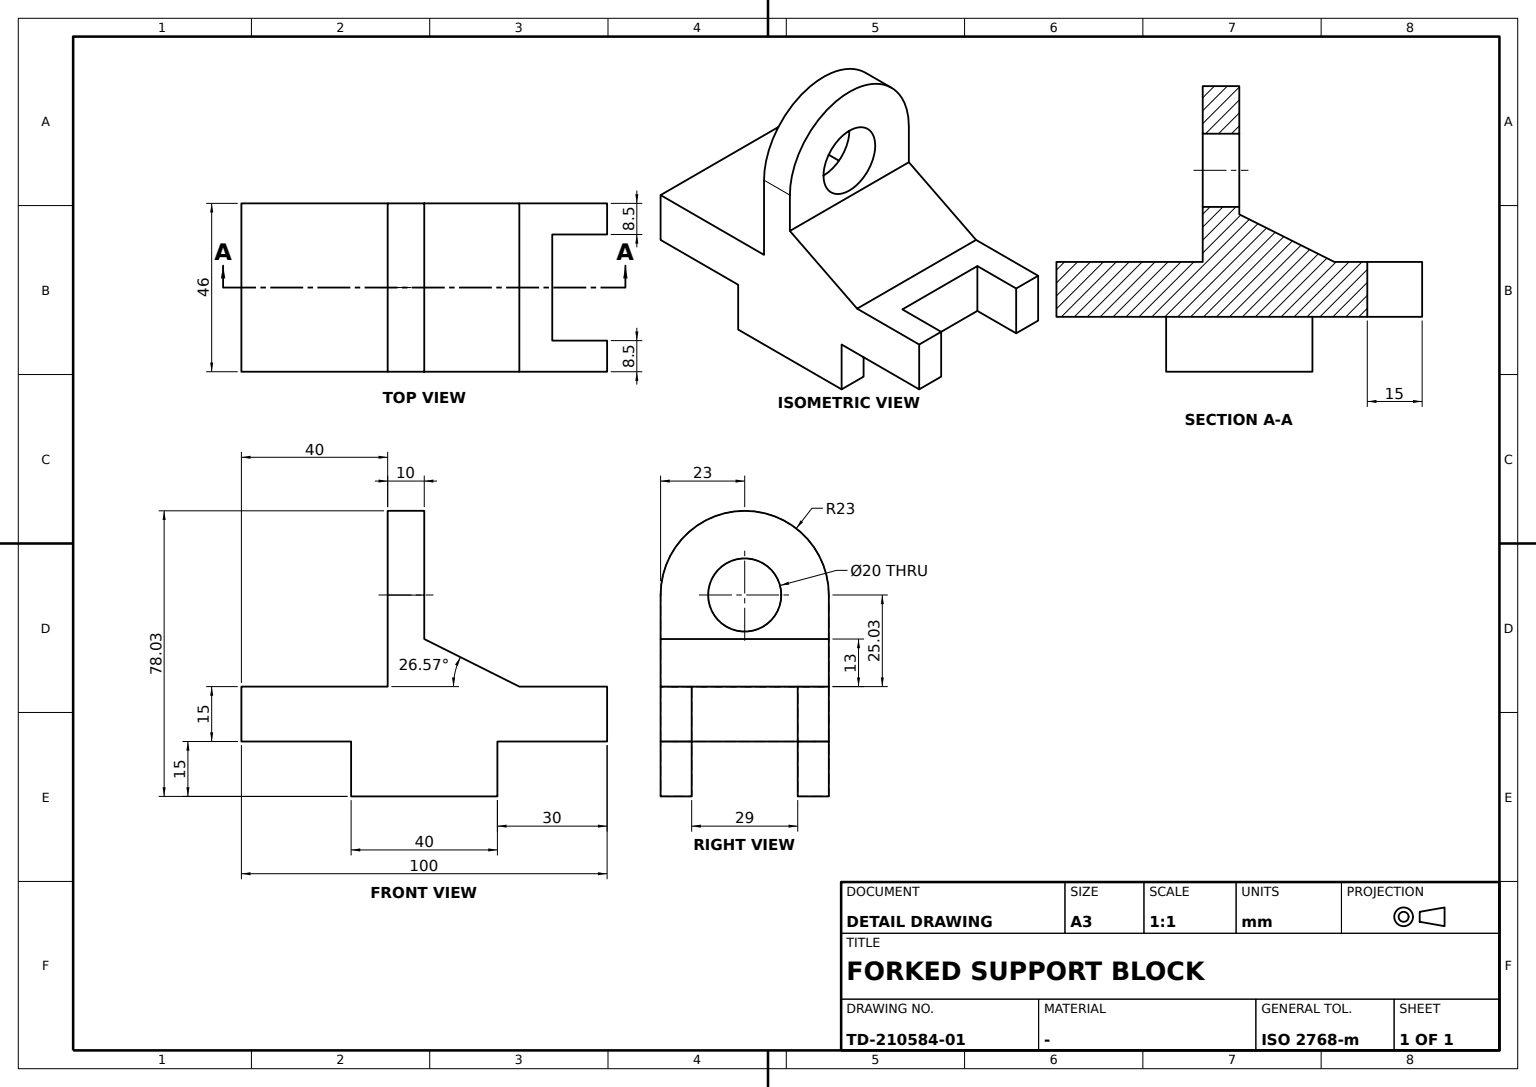
CATIA V5 part; units mm, degrees
sketch "Sketch1" plane through (0, 0, 0) normal (0, 1, 0) x (-1, 0, 0)
  line L0 (-20, 0) -> (20, 0)
  line L1 (20, 0) -> (20, 15)
  line L2 (20, 15) -> (50, 15)
  point P0 (50, 15)
  line L3 (-20, 0) -> (-20, 15)
  point P1 (-20, 15)
  line L4 (-20, 15) -> (-50, 15)
  point P2 (-50, 15)
  line L5 (-50, 15) -> (-50, 30)
  line L6 (-50, 30) -> (-26, 30)
  line L7 (50, 15) -> (50, 30)
  line L8 (50, 30) -> (10, 30)
  line L9 (10, 30) -> (10, 55)
  point P3 (10, 55)
  line L10 (10, 55) -> (0, 55)
  line L11 (0, 55) -> (0, 43)
  point P4 (0, 43)
  line L12 (-26, 30) -> (0, 43)
  dimension "length L0" = 40
  dimension "length L1" = 15
  dimension "length L2" = 30
  dimension "distance P2 P0" = 100
  dimension "length L5" = 15
  dimension "length L6" = 24
  dimension "length L7" = 15
  dimension "length L8" = 40
  dimension "distance P3 L0" = 55
  dimension "length L10" = 10
  dimension "distance P4 L8" = 13
  constraint midpoint L0 origin
  constraint horizontal L0 x-axis
  constraint horizontal L2 x-axis
  constraint horizontal L4 x-axis
  constraint horizontal L6 x-axis
  constraint horizontal L8 x-axis
  constraint horizontal L10 x-axis
  constraint vertical L1 y-axis
  constraint vertical L3 y-axis
  constraint vertical L5 y-axis
  constraint vertical L7 y-axis
  constraint vertical L9 y-axis
  constraint vertical L11 y-axis
  constraint coincidence P1 L2
extrude "Pad1" add sketch "Sketch1" along normal mid plane 46
sketch "Sketch2" plane through (0, 0, 0) normal (1, 0, 0) x (0, 1, 0)
  point P0 (-23, 55)
  arc A0 (-23, 55) -> (23, 55) centre (0, 55.0343) cw
  line L0 (-23, 55) -> (23, 55)
  line L1 (-23, 55) -> (-23, 43) construction
  dimension "radius A0" = 23
  dimension "length L0" = 46
  dimension "distance L0 x axis" = 55
  constraint horizontal L0 x-axis
  constraint coincidence P0 L1
extrude "Pad2" add sketch "Sketch2" against normal blind 10
sketch "Sketch3" plane through (0, 0, 0) normal (1, 0, 0) x (0, 1, 0)
  circle A0 centre (0, 55.0343) radius 10
  arc A1 (23, 55) -> (-23, 55) centre (0, 55.0343) ccw construction
  dimension "radius A0" = 10
  constraint concentricity A0 A1
extrude "Pocket1" cut sketch "Sketch3" against normal blind 10
sketch "Sketch4" plane through (-20, 0, 0) normal (-1, 0, 0) x (0, -1, 0)
  point P0 (0, 7.5)
  line L0 (14.5, 15) -> (14.5, 0)
  line L1 (14.5, 0) -> (-14.5, 0)
  line L2 (-14.5, 0) -> (-14.5, 15)
  line L3 (-14.5, 15) -> (14.5, 15)
  line L4 (23, 0) -> (-23, 0) construction
  dimension "length L1" = 29
  dimension "length L0" = 15
  constraint coincidence P0 y-axis
  constraint coincidence L1 L4
  constraint vertical L0 y-axis
  constraint vertical L2 y-axis
  constraint horizontal L1 x-axis
  constraint horizontal L3 x-axis
  constraint equidistance L0 L2 P0
  constraint equidistance L1 L3 P0
extrude "Pocket2" cut sketch "Sketch4" against normal through all
sketch "Sketch5" plane through (0, 0, 30) normal (0, 0, 1) x (1, 0, 0)
  point P0 (42.5, 0)
  line L0 (50, 14.5) -> (50, -14.5)
  line L1 (50, -14.5) -> (35, -14.5)
  line L2 (35, -14.5) -> (35, 14.5)
  line L3 (35, 14.5) -> (50, 14.5)
  line L4 (50, -23) -> (50, 23) construction
  dimension "length L0" = 29
  dimension "length L1" = 15
  constraint coincidence P0 x-axis
  constraint coincidence L0 L4
  constraint vertical L0 y-axis
  constraint vertical L2 y-axis
  constraint horizontal L1 x-axis
  constraint horizontal L3 x-axis
  constraint equidistance L0 L2 P0
  constraint equidistance L1 L3 P0
extrude "Pocket3" cut sketch "Sketch5" against normal through all
